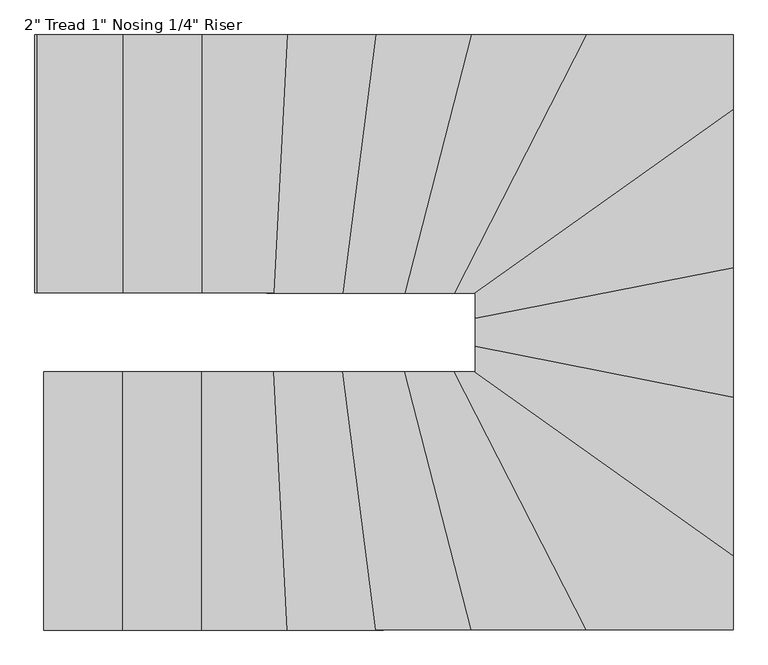
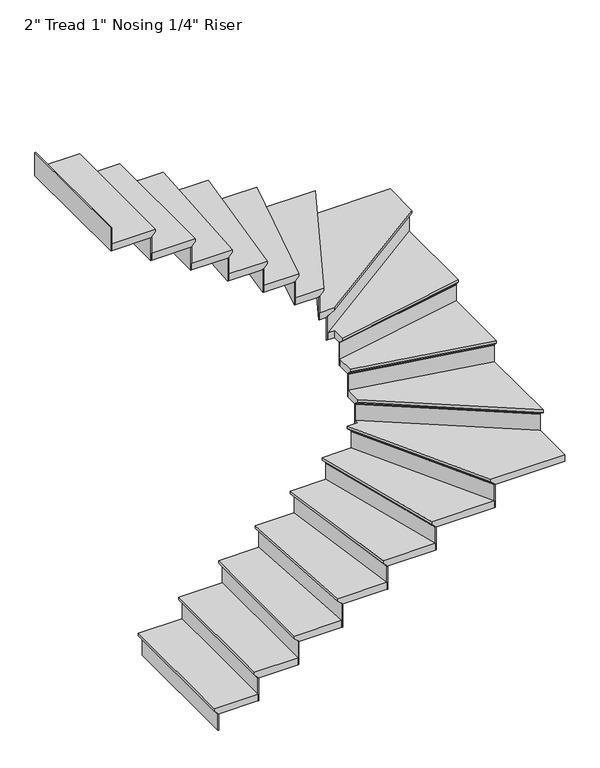
"""IFC4 building model written with IfcOpenShell, lengths in millimetres: stair flight geometry."""

from ifc_helpers import new_model, si_unit, origin, place, context, project, spatial, faceted_brep, source, transform, mapped, element, save


def stair_flight_8f30da42(model_context):
    return source(origin(), model_context, "Body", "Brep", [
        faceted_brep([(531.7538115, -7565.2090409, 6551.0833333), (531.7538115, -7565.2090409, 6570.1333333), (531.7538115, -6650.8090409, 6570.1333333), (531.7538115, -6650.8090409, 6551.0833333), (557.1538115, -7565.2090409, 6525.6833333), (557.1538115, -6650.8090409, 6525.6833333), (836.5538115, -7565.2090409, 6570.1333333), (836.5538115, -6650.8090409, 6570.1333333), (557.1538115, -6650.8090409, 6519.3333333), (836.5538115, -6650.8090409, 6519.3333333), (836.5538115, -7565.2090409, 6519.3333333), (557.1538115, -7565.2090409, 6519.3333333)], [[[0, 1, 2, 3]], [[4, 0, 3, 5]], [[2, 1, 6, 7]], [[8, 9, 10, 11]], [[2, 7, 9, 8, 5, 3]], [[8, 11, 4, 5]], [[6, 1, 0, 4, 11, 10]], [[7, 6, 10, 9]]]),
        faceted_brep([(557.1538115, -7565.2090409, 6519.3333333), (557.1538115, -7565.2090409, 6400.8), (563.5038115, -7565.2090409, 6400.8), (563.5038115, -7565.2090409, 6519.3333333), (557.1538115, -6650.8090409, 6519.3333333), (563.5038115, -6650.8090409, 6519.3333333), (563.5038115, -6650.8090409, 6400.8), (557.1538115, -6650.8090409, 6400.8)], [[[0, 1, 2, 3]], [[4, 5, 6, 7]], [[1, 0, 4, 7]], [[2, 1, 7, 6]], [[3, 2, 6, 5]], [[0, 3, 5, 4]]]),
        faceted_brep([(836.5538115, -7565.2090409, 6688.6666667), (836.5538115, -7565.2090409, 6519.3333333), (842.9038115, -7565.2090409, 6519.3333333), (842.9038115, -7565.2090409, 6688.6666667), (836.5538115, -6650.8090409, 6688.6666667), (842.9038115, -6650.8090409, 6688.6666667), (842.9038115, -6650.8090409, 6519.3333333), (836.5538115, -6650.8090409, 6519.3333333)], [[[0, 1, 2, 3]], [[4, 5, 6, 7]], [[1, 0, 4, 7]], [[2, 1, 7, 6]], [[3, 2, 6, 5]], [[0, 3, 5, 4]]]),
        faceted_brep([(811.1538115, -6650.8090409, 6739.4666667), (811.1538115, -7565.2090409, 6739.4666667), (1115.9538115, -7565.2090409, 6739.4666667), (1115.9538115, -6650.8090409, 6739.4666667), (836.5538115, -6650.8090409, 6688.6666667), (1115.9538115, -6650.8090409, 6688.6666667), (1115.9538115, -7565.2090409, 6688.6666667), (836.5538115, -7565.2090409, 6688.6666667), (836.5538115, -6650.8090409, 6695.0166667), (811.1538115, -6650.8090409, 6720.4166667), (836.5538115, -7565.2090409, 6695.0166667), (811.1538115, -7565.2090409, 6720.4166667)], [[[0, 1, 2, 3]], [[4, 5, 6, 7]], [[0, 3, 5, 4, 8, 9]], [[4, 7, 10, 8]], [[2, 1, 11, 10, 7, 6]], [[3, 2, 6, 5]], [[11, 1, 0, 9]], [[10, 11, 9, 8]]]),
        faceted_brep([(1115.9538115, -7565.2090409, 6858.0), (1115.9538115, -7565.2090409, 6688.6666667), (1122.3038115, -7565.2090409, 6688.6666667), (1122.3038115, -7565.2090409, 6858.0), (1115.9538115, -6650.8090409, 6858.0), (1122.3038115, -6650.8090409, 6858.0), (1122.3038115, -6650.8090409, 6688.6666667), (1115.9538115, -6650.8090409, 6688.6666667)], [[[0, 1, 2, 3]], [[4, 5, 6, 7]], [[1, 0, 4, 7]], [[2, 1, 7, 6]], [[3, 2, 6, 5]], [[0, 3, 5, 4]]]),
        faceted_brep([(1090.5538115, -6650.8090409, 6908.8), (1090.5538115, -7565.2090409, 6908.8), (1419.1552434, -7565.2090409, 6908.8), (1371.620973, -6650.8090409, 6908.8), (1115.9538115, -6650.8090409, 6858.0), (1371.620973, -6650.8090409, 6858.0), (1419.1552434, -7565.2090409, 6858.0), (1115.9538115, -7565.2090409, 6858.0), (1115.9538115, -6650.8090409, 6864.35), (1090.5538115, -6650.8090409, 6889.75), (1115.9538115, -7565.2090409, 6864.35), (1090.5538115, -7565.2090409, 6889.75)], [[[0, 1, 2, 3]], [[4, 5, 6, 7]], [[0, 3, 5, 4, 8, 9]], [[4, 7, 10, 8]], [[2, 1, 11, 10, 7, 6]], [[3, 2, 6, 5]], [[11, 1, 0, 9]], [[10, 11, 9, 8]]]),
        faceted_brep([(1419.1552434, -7565.2090409, 7027.3333333), (1419.1552434, -7565.2090409, 6858.0), (1425.5138176, -7565.2090409, 6858.0), (1425.5138176, -7565.2090409, 7027.3333333), (1371.620973, -6650.8090409, 7027.3333333), (1377.9795471, -6650.8090409, 7027.3333333), (1377.9795471, -6650.8090409, 6858.0), (1371.620973, -6650.8090409, 6858.0)], [[[0, 1, 2, 3]], [[4, 5, 6, 7]], [[1, 0, 4, 7]], [[2, 1, 7, 6]], [[3, 2, 6, 5]], [[0, 3, 5, 4]]]),
        faceted_brep([(1346.1866763, -6650.8090409, 7078.1333333), (1393.7209467, -7565.2090409, 7078.1333333), (1734.1437245, -7565.2090409, 7078.1333333), (1615.7876728, -6650.8090409, 7078.1333333), (1371.620973, -6650.8090409, 7027.3333333), (1615.7876728, -6650.8090409, 7027.3333333), (1734.1437245, -7565.2090409, 7027.3333333), (1419.1552434, -7565.2090409, 7027.3333333), (1371.620973, -6650.8090409, 7033.6833333), (1346.1866763, -6650.8090409, 7059.0833333), (1419.1552434, -7565.2090409, 7033.6833333), (1393.7209467, -7565.2090409, 7059.0833333)], [[[0, 1, 2, 3]], [[4, 5, 6, 7]], [[0, 3, 5, 4, 8, 9]], [[4, 7, 10, 8]], [[2, 1, 11, 10, 7, 6]], [[3, 2, 6, 5]], [[11, 1, 0, 9]], [[10, 11, 9, 8]]]),
        faceted_brep([(1734.1437245, -7565.2090409, 7196.6666667), (1734.1437245, -7565.2090409, 7027.3333333), (1740.5466962, -7565.2090409, 7027.3333333), (1740.5466962, -7565.2090409, 7196.6666667), (1615.7876728, -6650.8090409, 7196.6666667), (1622.1906446, -6650.8090409, 7196.6666667), (1622.1906446, -6650.8090409, 7027.3333333), (1615.7876728, -6650.8090409, 7027.3333333)], [[[0, 1, 2, 3]], [[4, 5, 6, 7]], [[1, 0, 4, 7]], [[2, 1, 7, 6]], [[3, 2, 6, 5]], [[0, 3, 5, 4]]]),
        faceted_brep([(1590.1757857, -6650.8090409, 7247.4666667), (1708.5318374, -7565.2090409, 7247.4666667), (2072.5453427, -7565.2090409, 7247.4666667), (1837.4148953, -6650.8090409, 7247.4666667), (1615.7876728, -6650.8090409, 7196.6666667), (1837.4148953, -6650.8090409, 7196.6666667), (2072.5453427, -7565.2090409, 7196.6666667), (1734.1437245, -7565.2090409, 7196.6666667), (1615.7876728, -6650.8090409, 7203.0166667), (1590.1757857, -6650.8090409, 7228.4166667), (1734.1437245, -7565.2090409, 7203.0166667), (1708.5318374, -7565.2090409, 7228.4166667)], [[[0, 1, 2, 3]], [[4, 5, 6, 7]], [[0, 3, 5, 4, 8, 9]], [[4, 7, 10, 8]], [[2, 1, 11, 10, 7, 6]], [[3, 2, 6, 5]], [[11, 1, 0, 9]], [[10, 11, 9, 8]]]),
        faceted_brep([(2072.5453427, -7565.2090409, 7366.0), (2072.5453427, -7565.2090409, 7196.6666667), (2079.1019196, -7565.2090409, 7196.6666667), (2079.1019196, -7565.2090409, 7366.0), (1837.4148953, -6650.8090409, 7366.0), (1843.9714722, -6650.8090409, 7366.0), (1843.9714722, -6650.8090409, 7196.6666667), (1837.4148953, -6650.8090409, 7196.6666667)], [[[0, 1, 2, 3]], [[4, 5, 6, 7]], [[1, 0, 4, 7]], [[2, 1, 7, 6]], [[3, 2, 6, 5]], [[0, 3, 5, 4]]]),
        faceted_brep([(1811.1885878, -6650.8090409, 7416.8), (2046.3190352, -7565.2090409, 7416.8), (2482.5861527, -7565.2090409, 7416.8), (2013.7615314, -6650.8090409, 7416.8), (1837.4148953, -6650.8090409, 7366.0), (2013.7615314, -6650.8090409, 7366.0), (2482.5861527, -7565.2090409, 7366.0), (2072.5453427, -7565.2090409, 7366.0), (1837.4148953, -6650.8090409, 7372.35), (1811.1885878, -6650.8090409, 7397.75), (2072.5453427, -7565.2090409, 7372.35), (2046.3190352, -7565.2090409, 7397.75)], [[[0, 1, 2, 3]], [[4, 5, 6, 7]], [[0, 3, 5, 4, 8, 9]], [[4, 7, 10, 8]], [[2, 1, 11, 10, 7, 6]], [[3, 2, 6, 5]], [[11, 1, 0, 9]], [[10, 11, 9, 8]]]),
        faceted_brep([(2482.5861527, -7565.2090409, 7535.3333333), (2482.5861527, -7565.2090409, 7366.0), (2489.7221358, -7565.2090409, 7366.0), (2489.7221358, -7565.2090409, 7535.3333333), (2013.7615314, -6650.8090409, 7535.3333333), (2020.8975145, -6650.8090409, 7535.3333333), (2020.8975145, -6650.8090409, 7366.0), (2013.7615314, -6650.8090409, 7366.0)], [[[0, 1, 2, 3]], [[4, 5, 6, 7]], [[1, 0, 4, 7]], [[2, 1, 7, 6]], [[3, 2, 6, 5]], [[0, 3, 5, 4]]]),
        faceted_brep([(2059.4855034, -6621.253958, 7586.1333333), (2059.4855034, -6650.8090409, 7586.1333333), (1985.2175988, -6650.8090409, 7586.1333333), (2454.0422202, -7565.2090409, 7586.1333333), (2973.8855034, -7565.2090409, 7586.1333333), (2973.8855034, -7271.5279072, 7586.1333333), (2059.4855034, -6650.8090409, 7535.3333333), (2059.4855034, -6621.253958, 7535.3333333), (2973.8855034, -7271.5279072, 7535.3333333), (2973.8855034, -7565.2090409, 7535.3333333), (2482.5861527, -7565.2090409, 7535.3333333), (2013.7615314, -6650.8090409, 7535.3333333), (2013.7615314, -6650.8090409, 7541.6833333), (1985.2175988, -6650.8090409, 7567.0833333), (2482.5861527, -7565.2090409, 7541.6833333), (2454.0422202, -7565.2090409, 7567.0833333)], [[[0, 1, 2, 3, 4, 5]], [[6, 7, 8, 9, 10, 11]], [[1, 0, 7, 6]], [[2, 1, 6, 11, 12, 13]], [[11, 10, 14, 12]], [[4, 3, 15, 14, 10, 9]], [[5, 4, 9, 8]], [[0, 5, 8, 7]], [[15, 3, 2, 13]], [[14, 15, 13, 12]]]),
        faceted_brep([(2973.8855034, -7271.5279072, 7704.6666667), (2973.8855034, -7271.5279072, 7535.3333333), (2973.8855034, -7263.7359324, 7535.3333333), (2973.8855034, -7263.7359324, 7704.6666667), (2059.4855034, -6621.253958, 7704.6666667), (2059.4855034, -6613.4619832, 7704.6666667), (2059.4855034, -6613.4619832, 7535.3333333), (2059.4855034, -6621.253958, 7535.3333333)], [[[0, 1, 2, 3]], [[4, 5, 6, 7]], [[1, 0, 4, 7]], [[2, 1, 7, 6]], [[3, 2, 6, 5]], [[0, 3, 5, 4]]]),
        faceted_brep([(2059.4855034, -6652.4218572, 7755.4666667), (2973.8855034, -7302.6958063, 7755.4666667), (2973.8855034, -6715.0407273, 7755.4666667), (2059.4855034, -6534.7998709, 7755.4666667), (2059.4855034, -6621.253958, 7704.6666667), (2059.4855034, -6534.7998709, 7704.6666667), (2973.8855034, -6715.0407273, 7704.6666667), (2973.8855034, -7271.5279072, 7704.6666667), (2059.4855034, -6621.253958, 7711.0166667), (2059.4855034, -6652.4218572, 7736.4166667), (2973.8855034, -7271.5279072, 7711.0166667), (2973.8855034, -7302.6958063, 7736.4166667)], [[[0, 1, 2, 3]], [[4, 5, 6, 7]], [[0, 3, 5, 4, 8, 9]], [[4, 7, 10, 8]], [[3, 2, 6, 5]], [[11, 1, 0, 9]], [[10, 11, 9, 8]], [[2, 1, 11, 10, 7, 6]]]),
        faceted_brep([(2973.8855034, -6715.0407273, 7874.0), (2973.8855034, -6715.0407273, 7704.6666667), (2973.8855034, -6708.5685418, 7704.6666667), (2973.8855034, -6708.5685418, 7874.0), (2059.4855034, -6534.7998709, 7874.0), (2059.4855034, -6528.3276855, 7874.0), (2059.4855034, -6528.3276855, 7704.6666667), (2059.4855034, -6534.7998709, 7704.6666667)], [[[0, 1, 2, 3]], [[4, 5, 6, 7]], [[1, 0, 4, 7]], [[2, 1, 7, 6]], [[3, 2, 6, 5]], [[0, 3, 5, 4]]]),
        faceted_brep([(2059.4855034, -6560.6886127, 7924.8), (2973.8855034, -6740.929469, 7924.8), (2973.8855034, -6255.3998709, 7924.8), (2059.4855034, -6435.6407273, 7924.8), (2059.4855034, -6534.7998709, 7874.0), (2059.4855034, -6435.6407273, 7874.0), (2973.8855034, -6255.3998709, 7874.0), (2973.8855034, -6715.0407273, 7874.0), (2059.4855034, -6534.7998709, 7880.35), (2059.4855034, -6560.6886127, 7905.75), (2973.8855034, -6715.0407273, 7880.35), (2973.8855034, -6740.929469, 7905.75)], [[[0, 1, 2, 3]], [[4, 5, 6, 7]], [[0, 3, 5, 4, 8, 9]], [[4, 7, 10, 8]], [[2, 1, 11, 10, 7, 6]], [[3, 2, 6, 5]], [[11, 1, 0, 9]], [[10, 11, 9, 8]]]),
        faceted_brep([(2973.8855034, -6255.3998709, 8043.3333333), (2973.8855034, -6255.3998709, 7874.0), (2973.8855034, -6248.9276855, 7874.0), (2973.8855034, -6248.9276855, 8043.3333333), (2059.4855034, -6435.6407273, 8043.3333333), (2059.4855034, -6429.1685418, 8043.3333333), (2059.4855034, -6429.1685418, 7874.0), (2059.4855034, -6435.6407273, 7874.0)], [[[0, 1, 2, 3]], [[4, 5, 6, 7]], [[1, 0, 4, 7]], [[2, 1, 7, 6]], [[3, 2, 6, 5]], [[0, 3, 5, 4]]]),
        faceted_brep([(2013.3900289, -6371.4090409, 8094.1333333), (2059.4855034, -6371.4090409, 8094.1333333), (2059.4855034, -6461.529469, 8094.1333333), (2973.8855034, -6281.2886127, 8094.1333333), (2973.8855034, -5688.3543762, 8094.1333333), (2059.4855034, -6371.4090409, 8043.3333333), (2013.3900289, -6371.4090409, 8043.3333333), (2973.8855034, -5688.3543762, 8043.3333333), (2973.8855034, -6255.3998709, 8043.3333333), (2059.4855034, -6435.6407273, 8043.3333333), (2973.8855034, -6255.3998709, 8049.6833333), (2059.4855034, -6435.6407273, 8049.6833333), (2973.8855034, -6281.2886127, 8075.0833333), (2059.4855034, -6461.529469, 8075.0833333)], [[[0, 1, 2, 3, 4]], [[5, 6, 7, 8, 9]], [[1, 0, 6, 5]], [[9, 8, 10, 11]], [[4, 3, 12, 10, 8, 7]], [[0, 4, 7, 6]], [[12, 3, 2, 13]], [[10, 12, 13, 11]], [[2, 1, 5, 9, 11, 13]]]),
        faceted_brep([(2973.8855034, -5688.3543762, 8212.6666667), (2973.8855034, -5688.3543762, 8043.3333333), (2973.8855034, -5680.5624014, 8043.3333333), (2973.8855034, -5680.5624014, 8212.6666667), (2013.3900289, -6371.4090409, 8212.6666667), (2002.4331364, -6371.4090409, 8212.6666667), (2002.4331364, -6371.4090409, 8043.3333333), (2013.3900289, -6371.4090409, 8043.3333333)], [[[0, 1, 2, 3]], [[4, 5, 6, 7]], [[1, 0, 4, 7]], [[2, 1, 7, 6]], [[3, 2, 6, 5]], [[0, 3, 5, 4]]]),
        faceted_brep([(2057.2175988, -6371.4090409, 8263.4666667), (2973.8855034, -5719.5222754, 8263.4666667), (2973.8855034, -5457.0090409, 8263.4666667), (2425.4982876, -5457.0090409, 8263.4666667), (1956.6736663, -6371.4090409, 8263.4666667), (2013.3900289, -6371.4090409, 8212.6666667), (1956.6736663, -6371.4090409, 8212.6666667), (2425.4982876, -5457.0090409, 8212.6666667), (2973.8855034, -5457.0090409, 8212.6666667), (2973.8855034, -5688.3543762, 8212.6666667), (2013.3900289, -6371.4090409, 8219.0166667), (2057.2175988, -6371.4090409, 8244.4166667), (2973.8855034, -5688.3543762, 8219.0166667), (2973.8855034, -5719.5222754, 8244.4166667)], [[[0, 1, 2, 3, 4]], [[5, 6, 7, 8, 9]], [[0, 4, 6, 5, 10, 11]], [[5, 9, 12, 10]], [[2, 1, 13, 12, 9, 8]], [[4, 3, 7, 6]], [[13, 1, 0, 11]], [[12, 13, 11, 10]], [[3, 2, 8, 7]]]),
        faceted_brep([(2425.4982876, -5457.0090409, 8382.0), (2425.4982876, -5457.0090409, 8212.6666667), (2418.3623045, -5457.0090409, 8212.6666667), (2418.3623045, -5457.0090409, 8382.0), (1956.6736663, -6371.4090409, 8382.0), (1949.5376832, -6371.4090409, 8382.0), (1949.5376832, -6371.4090409, 8212.6666667), (1956.6736663, -6371.4090409, 8212.6666667)], [[[0, 1, 2, 3]], [[4, 5, 6, 7]], [[1, 0, 4, 7]], [[2, 1, 7, 6]], [[3, 2, 6, 5]], [[0, 3, 5, 4]]]),
        faceted_brep([(1985.2175988, -6371.4090409, 8432.8), (2454.0422202, -5457.0090409, 8432.8), (2020.0927278, -5457.0090409, 8432.8), (1784.9622804, -6371.4090409, 8432.8), (1956.6736663, -6371.4090409, 8382.0), (1784.9622804, -6371.4090409, 8382.0), (2020.0927278, -5457.0090409, 8382.0), (2425.4982876, -5457.0090409, 8382.0), (1956.6736663, -6371.4090409, 8388.35), (1985.2175988, -6371.4090409, 8413.75), (2425.4982876, -5457.0090409, 8388.35), (2454.0422202, -5457.0090409, 8413.75)], [[[0, 1, 2, 3]], [[4, 5, 6, 7]], [[0, 3, 5, 4, 8, 9]], [[4, 7, 10, 8]], [[2, 1, 11, 10, 7, 6]], [[3, 2, 6, 5]], [[11, 1, 0, 9]], [[10, 11, 9, 8]]]),
        faceted_brep([(2020.0927278, -5457.0090409, 8551.3333333), (2020.0927278, -5457.0090409, 8382.0), (2013.5361509, -5457.0090409, 8382.0), (2013.5361509, -5457.0090409, 8551.3333333), (1784.9622804, -6371.4090409, 8551.3333333), (1778.4057035, -6371.4090409, 8551.3333333), (1778.4057035, -6371.4090409, 8382.0), (1784.9622804, -6371.4090409, 8382.0)], [[[0, 1, 2, 3]], [[4, 5, 6, 7]], [[1, 0, 4, 7]], [[2, 1, 7, 6]], [[3, 2, 6, 5]], [[0, 3, 5, 4]]]),
        faceted_brep([(1811.1885878, -6371.4090409, 8602.1333333), (2046.3190352, -5457.0090409, 8602.1333333), (1682.9199502, -5457.0090409, 8602.1333333), (1564.5638986, -6371.4090409, 8602.1333333), (1784.9622804, -6371.4090409, 8551.3333333), (1564.5638986, -6371.4090409, 8551.3333333), (1682.9199502, -5457.0090409, 8551.3333333), (2020.0927278, -5457.0090409, 8551.3333333), (1784.9622804, -6371.4090409, 8557.6833333), (1811.1885878, -6371.4090409, 8583.0833333), (2020.0927278, -5457.0090409, 8557.6833333), (2046.3190352, -5457.0090409, 8583.0833333)], [[[0, 1, 2, 3]], [[4, 5, 6, 7]], [[0, 3, 5, 4, 8, 9]], [[4, 7, 10, 8]], [[2, 1, 11, 10, 7, 6]], [[3, 2, 6, 5]], [[11, 1, 0, 9]], [[10, 11, 9, 8]]]),
        faceted_brep([(1682.9199502, -5457.0090409, 8720.6666667), (1682.9199502, -5457.0090409, 8551.3333333), (1676.5169785, -5457.0090409, 8551.3333333), (1676.5169785, -5457.0090409, 8720.6666667), (1564.5638986, -6371.4090409, 8720.6666667), (1558.1609268, -6371.4090409, 8720.6666667), (1558.1609268, -6371.4090409, 8551.3333333), (1564.5638986, -6371.4090409, 8551.3333333)], [[[0, 1, 2, 3]], [[4, 5, 6, 7]], [[1, 0, 4, 7]], [[2, 1, 7, 6]], [[3, 2, 6, 5]], [[0, 3, 5, 4]]]),
        faceted_brep([(1590.1757857, -6371.4090409, 8771.4666667), (1708.5318374, -5457.0090409, 8771.4666667), (1368.2866501, -5457.0090409, 8771.4666667), (1320.7523797, -6371.4090409, 8771.4666667), (1564.5638986, -6371.4090409, 8720.6666667), (1320.7523797, -6371.4090409, 8720.6666667), (1368.2866501, -5457.0090409, 8720.6666667), (1682.9199502, -5457.0090409, 8720.6666667), (1564.5638986, -6371.4090409, 8727.0166667), (1590.1757857, -6371.4090409, 8752.4166667), (1682.9199502, -5457.0090409, 8727.0166667), (1708.5318374, -5457.0090409, 8752.4166667)], [[[0, 1, 2, 3]], [[4, 5, 6, 7]], [[0, 3, 5, 4, 8, 9]], [[4, 7, 10, 8]], [[2, 1, 11, 10, 7, 6]], [[3, 2, 6, 5]], [[11, 1, 0, 9]], [[10, 11, 9, 8]]]),
        faceted_brep([(1368.2866501, -5457.0090409, 8890.0), (1368.2866501, -5457.0090409, 8720.6666667), (1361.9280759, -5457.0090409, 8720.6666667), (1361.9280759, -5457.0090409, 8890.0), (1320.7523797, -6371.4090409, 8890.0), (1314.3938055, -6371.4090409, 8890.0), (1314.3938055, -6371.4090409, 8720.6666667), (1320.7523797, -6371.4090409, 8720.6666667)], [[[0, 1, 2, 3]], [[4, 5, 6, 7]], [[1, 0, 4, 7]], [[2, 1, 7, 6]], [[3, 2, 6, 5]], [[0, 3, 5, 4]]]),
        faceted_brep([(1346.1866763, -6371.4090409, 8940.8), (1393.7209467, -5457.0090409, 8940.8), (1065.1538115, -5457.0090409, 8940.8), (1065.1538115, -6371.4090409, 8940.8), (1320.7523797, -6371.4090409, 8890.0), (1065.1538115, -6371.4090409, 8890.0), (1065.1538115, -5457.0090409, 8890.0), (1368.2866501, -5457.0090409, 8890.0), (1320.7523797, -6371.4090409, 8896.35), (1346.1866763, -6371.4090409, 8921.75), (1368.2866501, -5457.0090409, 8896.35), (1393.7209467, -5457.0090409, 8921.75)], [[[0, 1, 2, 3]], [[4, 5, 6, 7]], [[0, 3, 5, 4, 8, 9]], [[4, 7, 10, 8]], [[2, 1, 11, 10, 7, 6]], [[3, 2, 6, 5]], [[11, 1, 0, 9]], [[10, 11, 9, 8]]]),
        faceted_brep([(1065.1538115, -5457.0090409, 9059.3333333), (1065.1538115, -5457.0090409, 8890.0), (1058.8038115, -5457.0090409, 8890.0), (1058.8038115, -5457.0090409, 9059.3333333), (1065.1538115, -6371.4090409, 9059.3333333), (1058.8038115, -6371.4090409, 9059.3333333), (1058.8038115, -6371.4090409, 8890.0), (1065.1538115, -6371.4090409, 8890.0)], [[[0, 1, 2, 3]], [[4, 5, 6, 7]], [[1, 0, 4, 7]], [[2, 1, 7, 6]], [[3, 2, 6, 5]], [[0, 3, 5, 4]]]),
        faceted_brep([(1090.5538115, -6371.4090409, 9110.1333333), (1090.5538115, -5457.0090409, 9110.1333333), (785.7538115, -5457.0090409, 9110.1333333), (785.7538115, -6371.4090409, 9110.1333333), (1065.1538115, -6371.4090409, 9059.3333333), (785.7538115, -6371.4090409, 9059.3333333), (785.7538115, -5457.0090409, 9059.3333333), (1065.1538115, -5457.0090409, 9059.3333333), (1065.1538115, -6371.4090409, 9065.6833333), (1090.5538115, -6371.4090409, 9091.0833333), (1065.1538115, -5457.0090409, 9065.6833333), (1090.5538115, -5457.0090409, 9091.0833333)], [[[0, 1, 2, 3]], [[4, 5, 6, 7]], [[0, 3, 5, 4, 8, 9]], [[4, 7, 10, 8]], [[2, 1, 11, 10, 7, 6]], [[3, 2, 6, 5]], [[11, 1, 0, 9]], [[10, 11, 9, 8]]]),
        faceted_brep([(785.7538115, -5457.0090409, 9228.6666667), (785.7538115, -5457.0090409, 9059.3333333), (779.4038115, -5457.0090409, 9059.3333333), (779.4038115, -5457.0090409, 9228.6666667), (785.7538115, -6371.4090409, 9228.6666667), (779.4038115, -6371.4090409, 9228.6666667), (779.4038115, -6371.4090409, 9059.3333333), (785.7538115, -6371.4090409, 9059.3333333)], [[[0, 1, 2, 3]], [[4, 5, 6, 7]], [[1, 0, 4, 7]], [[2, 1, 7, 6]], [[3, 2, 6, 5]], [[0, 3, 5, 4]]]),
        faceted_brep([(506.3538115, -5457.0090409, 9398.0), (506.3538115, -5457.0090409, 9228.6666667), (500.0038115, -5457.0090409, 9228.6666667), (500.0038115, -5457.0090409, 9398.0), (506.3538115, -6371.4090409, 9398.0), (500.0038115, -6371.4090409, 9398.0), (500.0038115, -6371.4090409, 9228.6666667), (506.3538115, -6371.4090409, 9228.6666667)], [[[0, 1, 2, 3]], [[4, 5, 6, 7]], [[1, 0, 4, 7]], [[2, 1, 7, 6]], [[3, 2, 6, 5]], [[0, 3, 5, 4]]]),
        faceted_brep([(811.1538115, -6371.4090409, 9279.4666667), (811.1538115, -5457.0090409, 9279.4666667), (506.3538115, -5457.0090409, 9279.4666667), (506.3538115, -6371.4090409, 9279.4666667), (785.7538115, -6371.4090409, 9228.6666667), (506.3538115, -6371.4090409, 9228.6666667), (506.3538115, -5457.0090409, 9228.6666667), (785.7538115, -5457.0090409, 9228.6666667), (785.7538115, -6371.4090409, 9235.0166667), (811.1538115, -6371.4090409, 9260.4166667), (785.7538115, -5457.0090409, 9235.0166667), (811.1538115, -5457.0090409, 9260.4166667)], [[[0, 1, 2, 3]], [[4, 5, 6, 7]], [[0, 3, 5, 4, 8, 9]], [[4, 7, 10, 8]], [[2, 1, 11, 10, 7, 6]], [[3, 2, 6, 5]], [[11, 1, 0, 9]], [[10, 11, 9, 8]]]),
    ])


if __name__ == "__main__":
    model = new_model("IFC4")
    model_context = context("Model", 3, world=origin())
    ifc_project = project(units=[si_unit("LENGTHUNIT", "METRE", prefix="MILLI")], contexts=[model_context])
    site = spatial("IfcSite", under=ifc_project)
    building = spatial("IfcBuilding", under=site)
    placement = place(None, origin())
    stair_flight_shape = stair_flight_8f30da42(model_context)
    element("IfcStairFlight", 1, ObjectType="2\" Tread 1\" Nosing 1/4\" Riser", at=placement, inside=building, context=model_context, shape_type="MappedRepresentation", body=[
        mapped(stair_flight_shape, transform((0.0, 0.0, 0.0), x_axis=(1.0, 0.0, 0.0), y_axis=(0.0, 1.0, 0.0), z_axis=(0.0, 0.0, 1.0))),
    ])
    save(model, "model.ifc")
